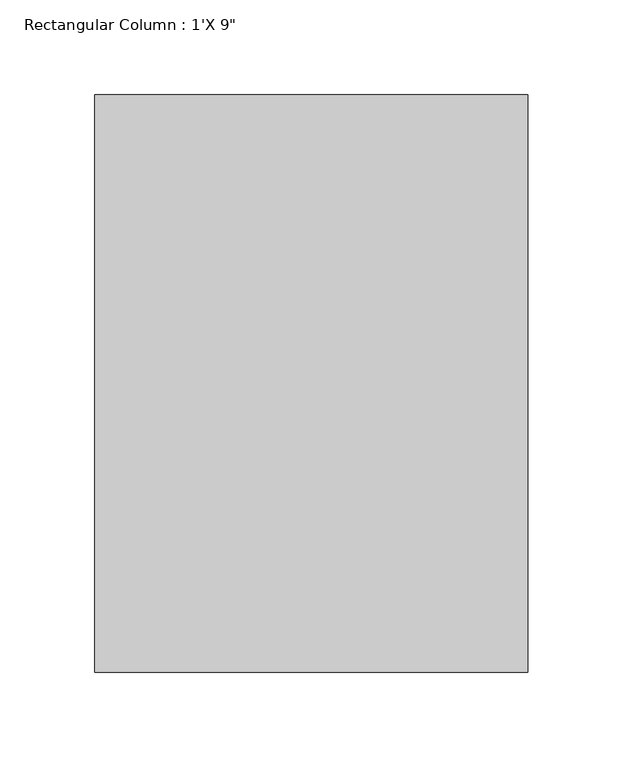
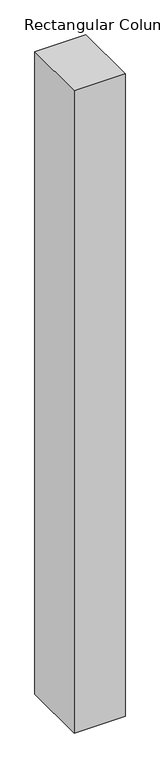
"""IFC4 building model written with IfcOpenShell, lengths in millimetres: column geometry."""

from ifc_helpers import new_model, si_unit, frame, origin, place, context, project, spatial, polyline, outline, extrude, source, transform, mapped, element, save


def column_216859a2(model_context):
    return source(origin(), model_context, "Body", "SweptSolid", [
        extrude(outline(polyline([(114.3, 152.4), (114.3, -152.4), (-114.3, -152.4), (-114.3, 152.4), (114.3, 152.4)])), frame((0.0, 0.0, 9601.2), z_axis=(0.0, 0.0, 1.0), x_axis=(1.0, 0.0, 0.0)), (0.0, 0.0, 1.0), 3048.0),
    ])


if __name__ == "__main__":
    model = new_model("IFC4")
    model_context = context("Model", 3, world=origin())
    ifc_project = project(units=[si_unit("LENGTHUNIT", "METRE", prefix="MILLI")], contexts=[model_context])
    site = spatial("IfcSite", under=ifc_project)
    building = spatial("IfcBuilding", under=site)
    placement = place(None, origin())
    column_shape = column_216859a2(model_context)
    element("IfcColumn", 1, ObjectType="Rectangular Column : 1'X 9\"", at=placement, inside=building, context=model_context, shape_type="MappedRepresentation", body=[
        mapped(column_shape, transform((0.0, 0.0, 0.0), x_axis=(1.0, 0.0, 0.0), y_axis=(0.0, 1.0, 0.0), z_axis=(0.0, 0.0, 1.0))),
    ])
    save(model, "model.ifc")

# Revit data of these elements
# Type "Rectangular Column : 1'X 9\""
#   Assembly Code = "B1010200"
#   Depth = 1' - 0"
#   Offset Base = 0' - 0"
#   Offset Top = 0' - 0"
#   Width = 0' - 9"
#   Material = none
